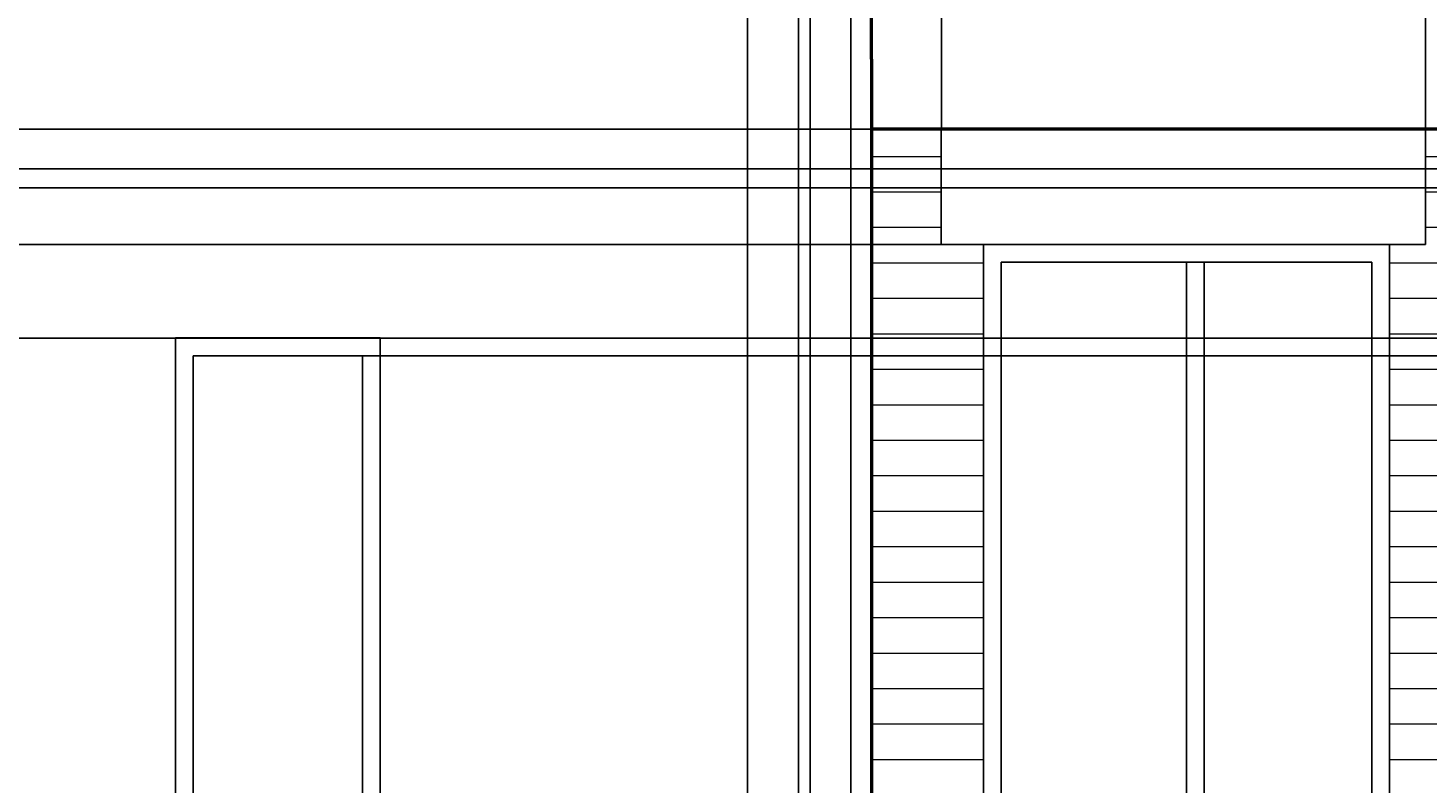
# Model space of a CAD drawing. Units: inches. Extents: x -139 to 346, y 72 to 413.
# Tile 4 of 18: x 18 to 175, y 157 to 242. Entities that reach past the tile are written whole.
import ezdxf

# ---------------------------------------------------------------- set-up
doc = ezdxf.new("R2010")
doc.units = ezdxf.units.IN
doc.header["$MEASUREMENT"] = 0
for name, color, linetype, lineweight in [('A-ANNO-DIMS', 2, 'Continuous', 18), ('A-DOOR', 3, 'Continuous', 25), ('A-ELEV', 9, 'Continuous', 25), ('A-GLAZ', 4, 'Continuous', 25), ('A-WALL', 7, 'Continuous', 50), ('A-WALL-PATT', 8, 'Continuous', 13)]:
    doc.layers.add(name, color=color, linetype=linetype, lineweight=lineweight)
doc.styles.get("Standard").update_dxf_attribs({"font": 'arial.ttf'})
doc.dimstyles.get("Standard").update_dxf_attribs({"dimtxt": 0.6875, "dimasz": 0.18, "dimexe": 0.18, "dimexo": 0.0625, "dimgap": 0.09, "dimtad": 0, "dimtih": 1, "dimtoh": 1, "dimdec": 4, "dimzin": 0, "dimdsep": 46, "dimlunit": 4, "dimtxsty": 'Standard', "dimcen": 0.09, "dimadec": 0, "dimazin": 0, "dimtfac": 1, "dimtdec": 4, "dimtofl": 0, "dimtmove": 0, "dimatfit": 3, "dimfxl": 1, "dimtolj": 1, "dimtzin": 0, "dimarcsym": 0})

# ---------------------------------------------------------------- blocks, each defined once
blk = doc.blocks.new('*D54')
at = {"layer": 'A-ANNO-DIMS', "color": 0, "lineweight": -2, "transparency": 16777216}
for p, q in [((-47.21, 224.46), (344.39, 224.46)), ((344.21, 224.28), (344.21, 216.43)), ((344.21, 207.7), (344.21, 215.55)), ((-47.21, 207.52), (344.39, 207.52))]:
    blk.add_line(p, q, dxfattribs=at)
at = {"layer": 'A-ANNO-DIMS', "color": 0, "transparency": 16777216}
for points in [[(344.18, 224.28), (344.24, 224.28), (344.21, 224.46)], [(344.18, 207.7), (344.24, 207.7), (344.21, 207.52)]]:
    blk.add_solid(points, dxfattribs=at)
at = {"layer": 'Defpoints', "color": 0, "transparency": 16777216}
for p in [(-47.27, 224.46), (344.21, 224.46), (-47.27, 207.52)]:
    blk.add_point(p, dxfattribs=at)
at = {"layer": 'A-ANNO-DIMS', "color": 0, "transparency": 16777216, "insert": (344.21, 215.99), "char_height": 0.688, "attachment_point": 5}
blk.add_mtext('\\A1;16.935', dxfattribs=at)
blk = doc.blocks.new('*D55')
at = {"layer": 'A-ANNO-DIMS', "color": 0, "lineweight": -2, "transparency": 16777216}
for p, q in [((-47.21, 226.61), (344.39, 226.61)), ((344.21, 226.43), (344.21, 225.97)), ((-47.21, 224.46), (344.39, 224.46)), ((344.21, 224.64), (344.21, 225.1))]:
    blk.add_line(p, q, dxfattribs=at)
at = {"layer": 'A-ANNO-DIMS', "color": 0, "transparency": 16777216}
for points in [[(344.18, 226.43), (344.24, 226.43), (344.21, 226.61)], [(344.18, 224.64), (344.24, 224.64), (344.21, 224.46)]]:
    blk.add_solid(points, dxfattribs=at)
at = {"layer": 'Defpoints', "color": 0, "transparency": 16777216}
for p in [(-47.27, 226.61), (344.21, 226.61), (-47.27, 224.46)]:
    blk.add_point(p, dxfattribs=at)
at = {"layer": 'A-ANNO-DIMS', "color": 0, "transparency": 16777216, "insert": (344.21, 225.53), "char_height": 0.688, "attachment_point": 5}
blk.add_mtext('\\A1;2.147', dxfattribs=at)
blk = doc.blocks.new('*D65')
at = {"layer": 'A-ANNO-DIMS', "color": 0, "lineweight": -2, "transparency": 16777216}
for p, q in [((55.33, 205.52), (344.39, 205.52)), ((344.21, 205.34), (344.21, 178.58)), ((344.21, 150.94), (344.21, 177.7)), ((55.33, 150.76), (344.39, 150.76))]:
    blk.add_line(p, q, dxfattribs=at)
at = {"layer": 'A-ANNO-DIMS', "color": 0, "transparency": 16777216}
for points in [[(344.18, 205.34), (344.24, 205.34), (344.21, 205.52)], [(344.18, 150.94), (344.24, 150.94), (344.21, 150.76)]]:
    blk.add_solid(points, dxfattribs=at)
at = {"layer": 'Defpoints', "color": 0, "transparency": 16777216}
for p in [(55.27, 205.52), (344.21, 205.52), (55.27, 150.76)]:
    blk.add_point(p, dxfattribs=at)
at = {"layer": 'A-ANNO-DIMS', "color": 0, "transparency": 16777216, "insert": (344.21, 178.14), "char_height": 0.688, "attachment_point": 5}
blk.add_mtext('\\A1;54.77', dxfattribs=at)
blk = doc.blocks.new('*D66')
at = {"layer": 'A-ANNO-DIMS', "color": 0, "lineweight": -2, "transparency": 16777216}
for p, q in [((57.33, 207.52), (344.39, 207.52)), ((344.21, 207.34), (344.21, 206.96)), ((55.33, 205.52), (344.39, 205.52)), ((344.21, 205.7), (344.21, 206.09))]:
    blk.add_line(p, q, dxfattribs=at)
at = {"layer": 'A-ANNO-DIMS', "color": 0, "transparency": 16777216}
for points in [[(344.18, 207.34), (344.24, 207.34), (344.21, 207.52)], [(344.18, 205.7), (344.24, 205.7), (344.21, 205.52)]]:
    blk.add_solid(points, dxfattribs=at)
at = {"layer": 'Defpoints', "color": 0, "transparency": 16777216}
for p in [(57.27, 207.52), (344.21, 207.52), (55.27, 205.52)]:
    blk.add_point(p, dxfattribs=at)
at = {"layer": 'A-ANNO-DIMS', "color": 0, "transparency": 16777216, "insert": (344.21, 206.52), "char_height": 0.688, "attachment_point": 5}
blk.add_mtext('\\A1;2', dxfattribs=at)
blk = doc.blocks.new('*D67')
at = {"layer": 'A-ANNO-DIMS', "color": 0, "lineweight": -2, "transparency": 16777216}
for p, q in [((57.33, 207.52), (344.39, 207.52)), ((344.21, 207.34), (344.21, 165.09)), ((344.21, 121.96), (344.21, 164.21)), ((57.33, 121.78), (344.39, 121.78))]:
    blk.add_line(p, q, dxfattribs=at)
at = {"layer": 'A-ANNO-DIMS', "color": 0, "transparency": 16777216}
for points in [[(344.18, 207.34), (344.24, 207.34), (344.21, 207.52)], [(344.18, 121.96), (344.24, 121.96), (344.21, 121.78)]]:
    blk.add_solid(points, dxfattribs=at)
at = {"layer": 'Defpoints', "color": 0, "transparency": 16777216}
for p in [(57.27, 207.52), (344.21, 207.52), (57.27, 121.78)]:
    blk.add_point(p, dxfattribs=at)
at = {"layer": 'A-ANNO-DIMS', "color": 0, "transparency": 16777216, "insert": (344.21, 164.65), "char_height": 0.688, "attachment_point": 5}
blk.add_mtext('\\A1;85.75', dxfattribs=at)
blk = doc.blocks.new('*D69')
at = {"layer": 'A-ANNO-DIMS', "color": 0, "lineweight": -2, "transparency": 16777216}
for p, q in [((120.51, 231.12), (120.51, 412.45)), ((120.69, 412.27), (146.54, 412.27)), ((174.89, 412.27), (149.04, 412.27)), ((175.07, 231.12), (175.07, 412.45))]:
    blk.add_line(p, q, dxfattribs=at)
at = {"layer": 'A-ANNO-DIMS', "color": 0, "transparency": 16777216}
for points in [[(120.69, 412.3), (120.69, 412.24), (120.51, 412.27)], [(174.89, 412.3), (174.89, 412.24), (175.07, 412.27)]]:
    blk.add_solid(points, dxfattribs=at)
at = {"layer": 'Defpoints', "color": 0, "transparency": 16777216}
for p in [(175.07, 412.27), (120.51, 231.06), (175.07, 231.06)]:
    blk.add_point(p, dxfattribs=at)
at = {"layer": 'A-ANNO-DIMS', "color": 0, "transparency": 16777216, "insert": (147.79, 412.27), "char_height": 0.688, "attachment_point": 5}
blk.add_mtext('\\A1;54.57', dxfattribs=at)
blk = doc.blocks.new('*D70')
at = {"layer": 'A-ANNO-DIMS', "color": 0, "lineweight": -2, "transparency": 16777216}
for p, q in [((125.18, 218.06), (-137.3, 218.06)), ((-137.12, 217.88), (-137.12, 167.31)), ((-137.12, 115.86), (-137.12, 166.43)), ((125.18, 115.68), (-137.3, 115.68))]:
    blk.add_line(p, q, dxfattribs=at)
at = {"layer": 'A-ANNO-DIMS', "color": 0, "transparency": 16777216}
for points in [[(-137.15, 217.88), (-137.09, 217.88), (-137.12, 218.06)], [(-137.15, 115.86), (-137.09, 115.86), (-137.12, 115.68)]]:
    blk.add_solid(points, dxfattribs=at)
at = {"layer": 'Defpoints', "color": 0, "transparency": 16777216}
for p in [(-137.12, 218.06), (125.25, 218.06), (125.25, 115.68)]:
    blk.add_point(p, dxfattribs=at)
at = {"layer": 'A-ANNO-DIMS', "color": 0, "transparency": 16777216, "insert": (-137.12, 166.87), "char_height": 0.688, "attachment_point": 5}
blk.add_mtext('\\A1;102.39', dxfattribs=at)
blk = doc.blocks.new('*D71')
at = {"layer": 'A-ANNO-DIMS', "color": 0, "lineweight": -2, "transparency": 16777216}
for p, q in [((120.44, 231.06), (-137.3, 231.06)), ((-137.12, 230.88), (-137.12, 225)), ((-137.12, 218.24), (-137.12, 224.12)), ((125.18, 218.06), (-137.3, 218.06))]:
    blk.add_line(p, q, dxfattribs=at)
at = {"layer": 'A-ANNO-DIMS', "color": 0, "transparency": 16777216}
for points in [[(-137.15, 230.88), (-137.09, 230.88), (-137.12, 231.06)], [(-137.15, 218.24), (-137.09, 218.24), (-137.12, 218.06)]]:
    blk.add_solid(points, dxfattribs=at)
at = {"layer": 'Defpoints', "color": 0, "transparency": 16777216}
for p in [(-137.12, 231.06), (120.51, 231.06), (125.25, 218.06)]:
    blk.add_point(p, dxfattribs=at)
at = {"layer": 'A-ANNO-DIMS', "color": 0, "transparency": 16777216, "insert": (-137.12, 224.56), "char_height": 0.688, "attachment_point": 5}
blk.add_mtext('\\A1;12.997', dxfattribs=at)
blk = doc.blocks.new('*D102')
at = {"layer": 'A-ANNO-DIMS', "color": 0, "lineweight": -2, "transparency": 16777216}
for p, q in [((98.67, 291), (98.67, 72.49)), ((104.42, 291), (104.42, 72.49)), ((98.85, 72.67), (100.3, 72.67)), ((104.24, 72.67), (102.79, 72.67))]:
    blk.add_line(p, q, dxfattribs=at)
at = {"layer": 'A-ANNO-DIMS', "color": 0, "transparency": 16777216}
for points in [[(98.85, 72.7), (98.85, 72.64), (98.67, 72.67)], [(104.24, 72.7), (104.24, 72.64), (104.42, 72.67)]]:
    blk.add_solid(points, dxfattribs=at)
at = {"layer": 'Defpoints', "color": 0, "transparency": 16777216}
for p in [(98.67, 291.06), (104.42, 291.06), (104.42, 72.67)]:
    blk.add_point(p, dxfattribs=at)
at = {"layer": 'A-ANNO-DIMS', "color": 0, "transparency": 16777216, "insert": (101.55, 72.67), "char_height": 0.688, "attachment_point": 5}
blk.add_mtext('\\A1;5.752', dxfattribs=at)
blk = doc.blocks.new('*D103')
at = {"layer": 'A-ANNO-DIMS', "color": 0, "lineweight": -2, "transparency": 16777216}
for p, q in [((104.42, 291), (104.42, 72.49)), ((105.74, 291), (105.74, 72.49)), ((104.6, 72.67), (105.56, 72.67)), ((105.74, 72.67), (105.92, 72.67))]:
    blk.add_line(p, q, dxfattribs=at)
at = {"layer": 'A-ANNO-DIMS', "color": 0, "transparency": 16777216}
for points in [[(104.6, 72.7), (104.6, 72.64), (104.42, 72.67)], [(105.56, 72.7), (105.56, 72.64), (105.74, 72.67)]]:
    blk.add_solid(points, dxfattribs=at)
at = {"layer": 'Defpoints', "color": 0, "transparency": 16777216}
for p in [(104.42, 291.06), (105.74, 291.06), (105.74, 72.67)]:
    blk.add_point(p, dxfattribs=at)
at = {"layer": 'A-ANNO-DIMS', "color": 0, "transparency": 16777216, "insert": (106.87, 72.67), "char_height": 0.688, "attachment_point": 5}
blk.add_mtext('\\A1;1.32', dxfattribs=at)
blk = doc.blocks.new('*D104')
at = {"layer": 'A-ANNO-DIMS', "color": 0, "lineweight": -2, "transparency": 16777216}
for p, q in [((110.32, 298.23), (110.32, 72.49)), ((105.74, 291), (105.74, 72.49)), ((105.92, 72.67), (106.77, 72.67)), ((110.14, 72.67), (109.29, 72.67))]:
    blk.add_line(p, q, dxfattribs=at)
at = {"layer": 'A-ANNO-DIMS', "color": 0, "transparency": 16777216}
for points in [[(105.92, 72.7), (105.92, 72.64), (105.74, 72.67)], [(110.14, 72.7), (110.14, 72.64), (110.32, 72.67)]]:
    blk.add_solid(points, dxfattribs=at)
at = {"layer": 'Defpoints', "color": 0, "transparency": 16777216}
for p in [(110.32, 298.29), (105.74, 291.06), (110.32, 72.67)]:
    blk.add_point(p, dxfattribs=at)
at = {"layer": 'A-ANNO-DIMS', "color": 0, "transparency": 16777216, "insert": (108.03, 72.67), "char_height": 0.688, "attachment_point": 5}
blk.add_mtext('\\A1;4.582', dxfattribs=at)
blk = doc.blocks.new('*D105')
at = {"layer": 'A-ANNO-DIMS', "color": 0, "lineweight": -2, "transparency": 16777216}
for p, q in [((110.32, 298.23), (110.32, 72.49)), ((112.65, 289), (112.65, 72.49)), ((110.5, 72.67), (112.47, 72.67)), ((112.65, 72.67), (112.83, 72.67))]:
    blk.add_line(p, q, dxfattribs=at)
at = {"layer": 'A-ANNO-DIMS', "color": 0, "transparency": 16777216}
for points in [[(110.5, 72.7), (110.5, 72.64), (110.32, 72.67)], [(112.47, 72.7), (112.47, 72.64), (112.65, 72.67)]]:
    blk.add_solid(points, dxfattribs=at)
at = {"layer": 'Defpoints', "color": 0, "transparency": 16777216}
for p in [(110.32, 298.29), (112.65, 289.06), (112.65, 72.67)]:
    blk.add_point(p, dxfattribs=at)
at = {"layer": 'A-ANNO-DIMS', "color": 0, "transparency": 16777216, "insert": (114.09, 72.67), "char_height": 0.688, "attachment_point": 5}
blk.add_mtext('\\A1;2.326', dxfattribs=at)

msp = doc.modelspace()

# ---------------------------------------------------------------- hatches: boundary and pattern name
at = {"layer": 'A-WALL-PATT'}
h = msp.add_hatch(dxfattribs=at)
h.set_pattern_fill('ANSI31', color=256, scale=32, angle=135)
h.paths.add_polyline_path([(98.6724, 360.5443), (-34.7346, 360.5443), (-34.7346, 353.0644), (-34.7346, 305.9205), (5.6729, 305.9205), (5.6729, 338.3217), (62.4258, 338.3217), (62.4258, 305.9205), (98.6724, 305.9205)])
h.paths.add_polyline_path([(212.769, 231.0607), (175.072, 231.0607), (175.072, 218.0635), (171.0337, 218.0635), (171.0337, 115.6761), (125.2464, 115.6761), (125.2464, 218.0635), (123.4318, 218.0635), (120.5054, 218.0635), (120.5054, 231.0607), (112.6506, 231.0607), (112.6506, 112.6042), (212.769, 112.6042)])

# ---------------------------------------------------------------- linework, layer by layer
at = {"layer": 'A-DOOR'}
for p, q in [((148.1401, 212.5413), (148.1401, 216.0635)), ((150.1401, 212.5413), (150.1401, 216.0635)), ((148.1401, 212.5413), (148.1401, 117.6761)), ((150.1401, 212.5413), (150.1401, 117.6761))]:
    msp.add_line(p, q, dxfattribs=at)
for points in [[(125.2464, 218.0635), (171.0337, 218.0635), (171.0337, 115.6761), (125.2464, 115.6761)], [(127.2464, 216.0635), (169.0337, 216.0635), (169.0337, 117.6761), (127.2464, 117.6761)]]:
    msp.add_lwpolyline(points, close=True, dxfattribs=at)
at = {"layer": 'A-ELEV'}
for p, q in [((120.5054, 231.0607), (120.5054, 218.0635)), ((175.072, 218.0635), (175.072, 231.0607)), ((120.5054, 218.0635), (123.4318, 218.0635)), ((123.4318, 218.0635), (125.2464, 218.0635)), ((171.0337, 218.0635), (175.072, 218.0635))]:
    msp.add_line(p, q, dxfattribs=at)
at = {"layer": 'A-GLAZ'}
for points in [[(34.1727, 207.5243), (57.2654, 207.5243), (57.2654, 121.7753), (34.1727, 121.7753)], [(36.1727, 205.5243), (55.2654, 205.5243), (55.2654, 123.7753), (36.1727, 123.7753)]]:
    msp.add_lwpolyline(points, close=True, dxfattribs=at)
at = {"layer": 'A-WALL'}
for p, q in [((112.6506, 238.9748), (112.6506, 274.9748)), ((112.6506, 238.9748), (112.6506, 94.9748)), ((297.5013, 231.0607), (112.6506, 231.0607))]:
    msp.add_line(p, q, dxfattribs=at)

# ---------------------------------------------------------------- dimensions: what is measured, and where the dimension line sits
at = {"layer": 'A-ANNO-DIMS'}
for base, p1, p2, override, picture, middle in [((175.072, 412.2748), (120.5054, 231.0607), (175.072, 231.0607), {"dimdec": 2, "dimlfac": 1, "dimrnd": 0, "dimzin": 0, "dimdsep": 46, "dimlunit": 2}, '*D69', (147.7887, 412.2748)), ((110.3243, 72.6748), (105.7421, 291.0604), (110.3243, 298.293), {"dimdec": 3, "dimlfac": 1, "dimrnd": 0, "dimzin": 0, "dimdsep": 46, "dimlunit": 2}, '*D104', (108.0332, 72.6748)), ((112.6506, 72.6748), (110.3243, 298.293), (112.6506, 289.0604), {"dimdec": 3, "dimlfac": 1, "dimrnd": 0, "dimzin": 0, "dimdsep": 46, "dimlunit": 2}, '*D105', (114.0862, 72.6748)), ((104.4244, 72.6748), (98.6724, 291.0604), (104.4244, 291.0604), {"dimdec": 3, "dimlfac": 1, "dimrnd": 0, "dimzin": 0, "dimdsep": 46, "dimlunit": 2}, '*D102', (101.5484, 72.6748)), ((105.7421, 72.6748), (104.4244, 291.0604), (105.7421, 291.0604), {"dimdec": 2, "dimlfac": 1, "dimrnd": 0, "dimzin": 0, "dimdsep": 46, "dimlunit": 2}, '*D103', (106.8691, 72.6748))]:
    dim = msp.add_linear_dim(base=base, p1=p1, p2=p2, dimstyle='Standard', override=override, dxfattribs=at)
    dim.commit()
    dim.dimension.update_dxf_attribs({"geometry": picture, "text_midpoint": middle})
for base, p1, p2, override, picture, middle in [((-137.1237, 231.0607), (125.2464, 218.0635), (120.5054, 231.0607), {"dimdec": 3, "dimlfac": 1, "dimrnd": 0, "dimzin": 0, "dimdsep": 46, "dimlunit": 2}, '*D71', (-137.1237, 224.5621)), ((344.2055, 226.6062), (-47.2734, 224.4591), (-47.2734, 226.6062), {"dimdec": 3, "dimlfac": 1, "dimrnd": 0, "dimzin": 0, "dimdsep": 46, "dimlunit": 2}, '*D55', (344.2055, 225.5327)), ((344.2055, 224.4591), (-47.2734, 207.5243), (-47.2734, 224.4591), {"dimdec": 3, "dimlfac": 1, "dimrnd": 0, "dimzin": 0, "dimdsep": 46, "dimlunit": 2}, '*D54', (344.2055, 215.9917)), ((-137.1237, 218.0635), (125.2464, 115.6761), (125.2464, 218.0635), {"dimdec": 2, "dimlfac": 1, "dimrnd": 0, "dimzin": 0, "dimdsep": 46, "dimlunit": 2}, '*D70', (-137.1237, 166.8698)), ((344.2055, 207.5243), (55.2654, 205.5243), (57.2654, 207.5243), {"dimdec": 0, "dimlfac": 1, "dimrnd": 0, "dimzin": 0, "dimdsep": 46, "dimlunit": 2}, '*D66', (344.2055, 206.5243)), ((344.2055, 207.5243), (57.2654, 121.7753), (57.2654, 207.5243), {"dimdec": 2, "dimlfac": 1, "dimrnd": 0, "dimzin": 0, "dimdsep": 46, "dimlunit": 2}, '*D67', (344.2055, 164.6498)), ((344.2055, 205.5243), (55.2654, 150.7576), (55.2654, 205.5243), {"dimdec": 2, "dimlfac": 1, "dimrnd": 0, "dimzin": 0, "dimdsep": 46, "dimlunit": 2}, '*D65', (344.2055, 178.141))]:
    dim = msp.add_linear_dim(base=base, p1=p1, p2=p2, angle=90, dimstyle='Standard', override=override, dxfattribs=at)
    dim.commit()
    dim.dimension.update_dxf_attribs({"geometry": picture, "text_midpoint": middle})

doc.saveas('drawing.dxf')
